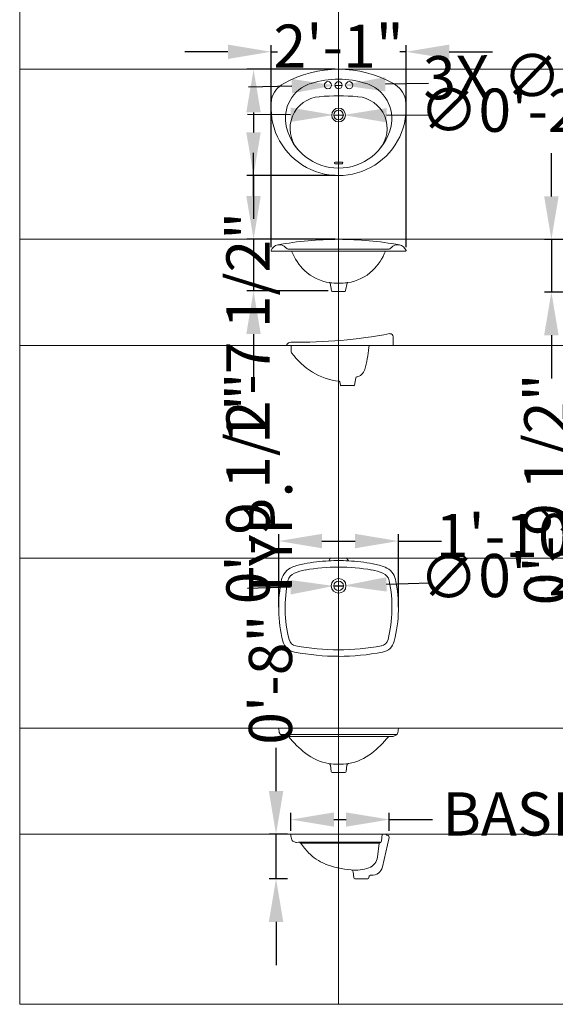
# Model space of a CAD drawing. Units: inches. Extents: x 2138 to 3265, y 2149 to 3392.
# Tile 7 of 13: x 2828 to 2928, y 3066 to 3248. Entities that reach past the tile are written whole.
import ezdxf

# ---------------------------------------------------------------- set-up
doc = ezdxf.new("R2010")
doc.units = ezdxf.units.IN
for name, color, linetype, lineweight in [('A-ANNO-DIMS', 2, 'Continuous', 18), ('A-DETL-GRID', 1, 'Continuous', 13), ('Washbasin-detail', 251, 'Continuous', 13), ('Washbasin-outline', 250, 'Continuous', 20)]:
    doc.layers.add(name, color=color, linetype=linetype, lineweight=lineweight)
doc.styles.get("Standard").update_dxf_attribs({"font": 'arial.ttf'})
doc.dimstyles.new('ISO-25', dxfattribs={"dimtxt": 8, "dimasz": 8, "dimexe": 1.25, "dimexo": 0.625, "dimtad": 0, "dimdec": 1, "dimlunit": 4, "dimtxsty": 'Standard', "dimcen": 2.5, "dimadec": 0, "dimazin": 0, "dimtfac": 1, "dimtdec": 1, "dimtmove": 0, "dimatfit": 3, "dimfxl": 1, "dimarcsym": 0})

# ---------------------------------------------------------------- blocks, each defined once
blk = doc.blocks.new('BASIN-WALLHUNG-SIDE')
for p, q in [((16.94, 8.23), (16.8, 6.96)), ((0.38, 6.97), (0.83, 6.75)), ((1.41, 6.77), (1.08, 6.71)), ((1.41, 6.77), (16.72, 6.77)), ((1.8, 6.61), (16.41, 6.61)), ((16.36, 6.61), (16.07, 4.02)), ((11.67, 0.17), (11.54, 1.3)), ((14.45, 0.17), (14.46, 0.29)), ((11.87, 0), (14.25, 0))]:
    blk.add_line(p, q)
for points in [[(17.61, 8.23), (0.08, 8.23, 0.427055), (0, 8.15, 0.060898), (0.18, 7.2)], [(17.81, 8.05), (18.01, 7.98, -0.38584), (18.2, 7.66), (16.99, 2.18)]]:
    blk.add_lwpolyline(points, format="xyb")
for centre, radius, start, end in [((17.61, 8.11), 0.119, 11.3189, 90), ((17.85, 8.16), 0.119, 191.3189, 251.9239), ((0.56, 7.33), 0.396, 197.6362, 243.4349), ((1.01, 7.1), 0.396, 243.4349, 279.8522), ((1.48, 6.38), 0.396, 36.3193, 99.8522), ((18.06, 18.57), 20.18, 216.3193, 223.028), ((16.41, 7.01), 0.396, 270, 353.6234), ((9.38, 10.47), 8.31, 223.028, 248.5761), ((13.71, 4.28), 2.37, 288.7646, 353.6234), ((12.27, 17.83), 16.23, 248.5761, 266.122), ((12.12, 7.8), 6.22, 261.2493, 292.2117), ((15.05, 2.61), 1.98, 265.1357, 347.5295), ((11.15, 1.25), 0.396, 6.7098, 86.122), ((11.87, 0.2), 0.198, 186.7098, 270), ((14.25, 0.2), 0.198, 270, 353.2902), ((14.85, 0.25), 0.396, 85.1357, 173.2902)]:
    blk.add_arc(centre, radius, start, end)
blk = doc.blocks.new('*D49')
at = {"layer": 'A-ANNO-DIMS', "color": 0, "lineweight": -2, "transparency": 16777216}
for p, q in [((2878.67, 3097.91), (2878.67, 3101.27)), ((2896.9, 3097.91), (2896.9, 3101.27)), ((2886.67, 3100.02), (2888.9, 3100.02)), ((2896.9, 3100.02), (2904.9, 3100.02))]:
    blk.add_line(p, q, dxfattribs=at)
at = {"layer": 'A-ANNO-DIMS', "color": 0, "transparency": 16777216}
for points in [[(2886.67, 3101.35), (2886.67, 3098.69), (2878.67, 3100.02)], [(2888.9, 3101.35), (2888.9, 3098.69), (2896.9, 3100.02)]]:
    blk.add_solid(points, dxfattribs=at)
at = {"layer": 'Defpoints', "color": 0, "transparency": 16777216}
for p in [(2896.9, 3100.02), (2878.67, 3097.29), (2896.9, 3097.29)]:
    blk.add_point(p, dxfattribs=at)
at = {"layer": 'A-ANNO-DIMS', "color": 0, "transparency": 16777216, "insert": (2948.05, 3100.02), "char_height": 8, "attachment_point": 5}
blk.add_mtext('BASIN 1\'-6" TYP.', dxfattribs=at)
blk = doc.blocks.new('*D50')
at = {"layer": 'A-ANNO-DIMS', "color": 0, "lineweight": -2, "transparency": 16777216}
for p, q in [((2875.94, 3105.29), (2875.94, 3113.29)), ((2878.04, 3097.29), (2874.69, 3097.29)), ((2875.94, 3089.06), (2875.94, 3097.29)), ((2878.04, 3089.06), (2874.69, 3089.06)), ((2875.94, 3081.06), (2875.94, 3073.06))]:
    blk.add_line(p, q, dxfattribs=at)
at = {"layer": 'A-ANNO-DIMS', "color": 0, "transparency": 16777216}
for points in [[(2874.6, 3105.29), (2877.27, 3105.29), (2875.94, 3097.29)], [(2874.6, 3081.06), (2877.27, 3081.06), (2875.94, 3089.06)]]:
    blk.add_solid(points, dxfattribs=at)
at = {"layer": 'Defpoints', "color": 0, "transparency": 16777216}
for p in [(2875.94, 3097.29), (2878.67, 3097.29), (2878.67, 3089.06)]:
    blk.add_point(p, dxfattribs=at)
at = {"layer": 'A-ANNO-DIMS', "color": 0, "transparency": 16777216, "insert": (2875.94, 3138.29), "char_height": 8, "attachment_point": 5, "rotation": 90}
blk.add_mtext('0\'-8" TYP.', dxfattribs=at)
blk = doc.blocks.new('*D79')
at = {"layer": 'A-ANNO-DIMS', "color": 0, "lineweight": -2, "transparency": 16777216}
for p, q in [((2875.02, 3206.04), (2875.02, 3243.52)), ((2900.02, 3206.04), (2900.02, 3243.52)), ((2867.02, 3242.27), (2859.02, 3242.27)), ((2875.02, 3242.27), (2876.19, 3242.27)), ((2900.02, 3242.27), (2898.84, 3242.27)), ((2908.02, 3242.27), (2916.02, 3242.27))]:
    blk.add_line(p, q, dxfattribs=at)
at = {"layer": 'A-ANNO-DIMS', "color": 0, "transparency": 16777216}
for points in [[(2867.02, 3243.6), (2867.02, 3240.94), (2875.02, 3242.27)], [(2908.02, 3243.6), (2908.02, 3240.94), (2900.02, 3242.27)]]:
    blk.add_solid(points, dxfattribs=at)
at = {"layer": 'Defpoints', "color": 0, "transparency": 16777216}
for p in [(2900.02, 3242.27), (2875.02, 3205.41), (2900.02, 3205.41)]:
    blk.add_point(p, dxfattribs=at)
at = {"layer": 'A-ANNO-DIMS', "color": 0, "transparency": 16777216, "insert": (2887.52, 3242.27), "char_height": 8, "attachment_point": 5}
blk.add_mtext('2\'-1"', dxfattribs=at)
blk = doc.blocks.new('*D80')
at = {"layer": 'A-ANNO-DIMS', "color": 0, "lineweight": -2, "transparency": 16777216}
for p, q in [((2886.89, 3239.02), (2870.52, 3239.02)), ((2871.77, 3231.02), (2871.77, 3227.33)), ((2886.89, 3219.33), (2870.52, 3219.33)), ((2871.77, 3219.33), (2871.77, 3211.33))]:
    blk.add_line(p, q, dxfattribs=at)
at = {"layer": 'A-ANNO-DIMS', "color": 0, "transparency": 16777216}
for points in [[(2870.43, 3231.02), (2873.1, 3231.02), (2871.77, 3239.02)], [(2870.43, 3227.33), (2873.1, 3227.33), (2871.77, 3219.33)]]:
    blk.add_solid(points, dxfattribs=at)
at = {"layer": 'Defpoints', "color": 0, "transparency": 16777216}
for p in [(2887.52, 3239.02), (2871.77, 3219.33), (2887.52, 3219.33)]:
    blk.add_point(p, dxfattribs=at)
at = {"layer": 'A-ANNO-DIMS', "color": 0, "transparency": 16777216, "insert": (2871.77, 3191.13), "char_height": 8, "attachment_point": 5, "rotation": 90}
blk.add_mtext('1\'-7 1/2"', dxfattribs=at)
blk = doc.blocks.new('*D81')
at = {"layer": 'A-ANNO-DIMS', "color": 0, "lineweight": -2, "transparency": 16777216}
for p, q in [((2871.77, 3215.52), (2871.77, 3223.52)), ((2886.89, 3207.52), (2870.52, 3207.52)), ((2871.77, 3207.52), (2871.77, 3197.95)), ((2885.61, 3197.95), (2870.52, 3197.95)), ((2871.77, 3189.95), (2871.77, 3181.95))]:
    blk.add_line(p, q, dxfattribs=at)
at = {"layer": 'A-ANNO-DIMS', "color": 0, "transparency": 16777216}
for points in [[(2870.43, 3215.52), (2873.1, 3215.52), (2871.77, 3207.52)], [(2870.43, 3189.95), (2873.1, 3189.95), (2871.77, 3197.95)]]:
    blk.add_solid(points, dxfattribs=at)
at = {"layer": 'Defpoints', "color": 0, "transparency": 16777216}
for p in [(2887.52, 3207.52), (2871.77, 3197.95), (2886.23, 3197.95)]:
    blk.add_point(p, dxfattribs=at)
at = {"layer": 'A-ANNO-DIMS', "color": 0, "transparency": 16777216, "insert": (2871.77, 3161.38), "char_height": 8, "attachment_point": 5, "rotation": 90}
blk.add_mtext('0\'-9 1/2"', dxfattribs=at)
blk = doc.blocks.new('*D83')
at = {"layer": 'A-ANNO-DIMS', "color": 0, "lineweight": -2, "transparency": 16777216}
for p, q in [((2926.93, 3215.47), (2926.93, 3223.47)), ((2930.28, 3207.47), (2925.68, 3207.47)), ((2926.93, 3207.47), (2926.93, 3197.76)), ((2946.5, 3197.76), (2925.68, 3197.76)), ((2926.93, 3189.76), (2926.93, 3181.76))]:
    blk.add_line(p, q, dxfattribs=at)
at = {"layer": 'A-ANNO-DIMS', "color": 0, "transparency": 16777216}
for points in [[(2925.59, 3215.47), (2928.26, 3215.47), (2926.93, 3207.47)], [(2925.59, 3189.76), (2928.26, 3189.76), (2926.93, 3197.76)]]:
    blk.add_solid(points, dxfattribs=at)
at = {"layer": 'Defpoints', "color": 0, "transparency": 16777216}
for p in [(2930.91, 3207.47), (2926.93, 3197.76), (2947.13, 3197.76)]:
    blk.add_point(p, dxfattribs=at)
at = {"layer": 'A-ANNO-DIMS', "color": 0, "transparency": 16777216, "insert": (2926.93, 3161.18), "char_height": 8, "attachment_point": 5, "rotation": 90}
blk.add_mtext('0\'-9 1/2"', dxfattribs=at)
blk = doc.blocks.new('*D97')
at = {"layer": 'A-ANNO-DIMS', "color": 0, "lineweight": -2, "transparency": 16777216}
for p, q in [((2876.44, 3139.39), (2876.44, 3152.87)), ((2898.59, 3139.39), (2898.59, 3152.87)), ((2884.44, 3151.62), (2890.59, 3151.62)), ((2898.59, 3151.62), (2906.59, 3151.62))]:
    blk.add_line(p, q, dxfattribs=at)
at = {"layer": 'A-ANNO-DIMS', "color": 0, "transparency": 16777216}
for points in [[(2884.44, 3152.95), (2884.44, 3150.28), (2876.44, 3151.62)], [(2890.59, 3152.95), (2890.59, 3150.28), (2898.59, 3151.62)]]:
    blk.add_solid(points, dxfattribs=at)
at = {"layer": 'Defpoints', "color": 0, "transparency": 16777216}
for p in [(2898.59, 3151.62), (2876.44, 3138.77), (2898.59, 3138.77)]:
    blk.add_point(p, dxfattribs=at)
at = {"layer": 'A-ANNO-DIMS', "color": 0, "transparency": 16777216, "insert": (2920.58, 3151.62), "char_height": 8, "attachment_point": 5}
blk.add_mtext('1\'-10"', dxfattribs=at)
blk = doc.blocks.new('*D121')
at = {"layer": 'A-ANNO-DIMS', "color": 0, "lineweight": -2, "transparency": 16777216}
for p, q in [((2904.18, 3236.4), (2896.19, 3236.24)), ((2878.85, 3235.89), (2870.85, 3235.74)), ((2886.85, 3236.05), (2888.19, 3236.08))]:
    blk.add_line(p, q, dxfattribs=at)
at = {"layer": 'A-ANNO-DIMS', "color": 0, "transparency": 16777216}
for points in [[(2878.82, 3237.23), (2878.88, 3234.56), (2886.85, 3236.05)], [(2896.16, 3237.57), (2896.21, 3234.91), (2888.19, 3236.08)]]:
    blk.add_solid(points, dxfattribs=at)
at = {"layer": 'Defpoints', "color": 0, "transparency": 16777216}
for p in [(2886.85, 3236.05), (2888.19, 3236.08)]:
    blk.add_point(p, dxfattribs=at)
at = {"layer": 'A-ANNO-DIMS', "color": 0, "transparency": 16777216, "insert": (2937.49, 3237.06), "char_height": 8, "attachment_point": 5, "rotation": 1.1379}
blk.add_mtext('3X ∅0\'-1 1/2"', dxfattribs=at)
blk = doc.blocks.new('*D122')
at = {"layer": 'A-ANNO-DIMS', "color": 0, "lineweight": -2, "transparency": 16777216}
for p, q in [((2878.63, 3230.6), (2870.63, 3230.64)), ((2886.63, 3230.56), (2888.4, 3230.55)), ((2904.4, 3230.47), (2896.4, 3230.51))]:
    blk.add_line(p, q, dxfattribs=at)
at = {"layer": 'A-ANNO-DIMS', "color": 0, "transparency": 16777216}
for points in [[(2878.64, 3231.93), (2878.63, 3229.27), (2886.63, 3230.56)], [(2896.41, 3231.84), (2896.4, 3229.18), (2888.4, 3230.55)]]:
    blk.add_solid(points, dxfattribs=at)
at = {"layer": 'Defpoints', "color": 0, "transparency": 16777216}
for p in [(2886.63, 3230.56), (2888.4, 3230.55)]:
    blk.add_point(p, dxfattribs=at)
at = {"layer": 'A-ANNO-DIMS', "color": 0, "transparency": 16777216, "insert": (2920.01, 3230.39), "char_height": 8, "attachment_point": 5, "rotation": 359.7153}
blk.add_mtext('∅0\'-2"', dxfattribs=at)
blk = doc.blocks.new('*D130')
at = {"layer": 'A-ANNO-DIMS', "color": 0, "lineweight": -2, "transparency": 16777216}
for p, q in [((2886.63, 3143.3), (2888.41, 3143.35)), ((2904.4, 3143.83), (2896.4, 3143.59)), ((2878.63, 3143.06), (2870.63, 3142.82))]:
    blk.add_line(p, q, dxfattribs=at)
at = {"layer": 'A-ANNO-DIMS', "color": 0, "transparency": 16777216}
for points in [[(2878.59, 3144.39), (2878.67, 3141.72), (2886.63, 3143.3)], [(2896.36, 3144.92), (2896.44, 3142.26), (2888.41, 3143.35)]]:
    blk.add_solid(points, dxfattribs=at)
at = {"layer": 'Defpoints', "color": 0, "transparency": 16777216}
for p in [(2886.63, 3143.3), (2888.41, 3143.35)]:
    blk.add_point(p, dxfattribs=at)
at = {"layer": 'A-ANNO-DIMS', "color": 0, "transparency": 16777216, "insert": (2920, 3144.3), "char_height": 8, "attachment_point": 5, "rotation": 1.7228}
blk.add_mtext('∅0\'-2"', dxfattribs=at)

msp = doc.modelspace()

# ---------------------------------------------------------------- linework, layer by layer
at = {"layer": 'A-DETL-GRID'}
for p, q in [((2828.46, 3239.02), (2828.46, 3370.91)), ((2887.52, 3239.02), (2887.52, 3370.91)), ((2828.46, 3239.02), (3241.85, 3239.02)), ((2828.46, 3239.02), (3241.85, 3239.02)), ((2828.46, 3148.47), (2828.46, 3239.02)), ((2887.52, 3148.47), (2887.52, 3239.02)), ((2828.46, 3207.52), (3241.85, 3207.52)), ((2828.46, 3187.84), (3241.85, 3187.84)), ((2828.46, 3148.47), (3241.85, 3148.47)), ((2828.46, 3148.47), (3241.85, 3148.47)), ((2828.46, 3065.79), (2828.46, 3148.47)), ((2887.52, 3065.79), (2887.52, 3148.47)), ((2828.46, 3116.97), (3241.85, 3116.97)), ((2828.46, 3097.29), (3241.85, 3097.29)), ((2828.46, 3065.79), (3241.85, 3065.79))]:
    msp.add_line(p, q, dxfattribs=at)
at = {"layer": 'Washbasin-detail'}
for p, q in [((2886.88, 3221.82), (2887.52, 3221.82)), ((2888.16, 3221.82), (2887.52, 3221.82)), ((2886.88, 3221.52), (2887.52, 3221.52)), ((2888.16, 3221.52), (2887.52, 3221.52)), ((2878.72, 3187.84), (2893.48, 3187.84)), ((2887.52, 3115.78), (2876.72, 3115.78)), ((2887.52, 3115.78), (2898.32, 3115.78))]:
    msp.add_line(p, q, dxfattribs=at)
for centre, radius in [((2885.55, 3236.07), 0.669), ((2887.52, 3236.07), 0.669), ((2889.49, 3236.07), 0.669), ((2887.52, 3230.55), 1.28), ((2887.52, 3230.55), 0.886), ((2887.52, 3143.32), 1.37), ((2887.52, 3143.32), 0.89)]:
    msp.add_circle(centre, radius, dxfattribs=at)
for centre, radius, start, end in [((2884.45, 3228.05), 5.92, 94.5762, 220.138), ((2887.52, 3189.71), 44.39, 85.4238, 94.5762), ((2890.59, 3228.05), 5.92, 319.862, 85.4238), ((2886.88, 3221.67), 0.146, 90, 270), ((2888.16, 3221.67), 0.146, 270, 90), ((2887.52, 3145.54), 61.98, 90, 100.4767), ((2887.52, 3145.54), 61.98, 79.5233, 90), ((2887.52, 3213.85), 14.46, 263.4006, 276.5994), ((2887.52, 3112.38), 34.43, 90, 100.3055), ((2887.52, 3112.38), 34.43, 79.6945, 90), ((2880.08, 3143.84), 1.98, 111.509, 168.1174), ((2883.27, 3135.74), 10.69, 100.3055, 111.509), ((2891.77, 3135.74), 10.69, 68.491, 79.6945), ((2894.96, 3143.84), 1.98, 11.8826, 68.491), ((2901.76, 3139.27), 24.14, 168.1174, 194.1676), ((2873.27, 3139.27), 24.14, 345.8324, 11.8826), ((2879.89, 3133.75), 1.58, 194.1676, 259.2192), ((2887.52, 3173.8), 42.34, 259.2192, 270), ((2887.52, 3173.8), 42.34, 270, 280.7808), ((2895.14, 3133.75), 1.58, 280.7808, 345.8324), ((2887.25, 3119.78), 9.5, 260.4365, 271.6387), ((2887.79, 3119.78), 9.5, 268.3613, 279.5635)]:
    msp.add_arc(centre, radius, start, end, dxfattribs=at)
at = {"layer": 'Washbasin-outline'}
for p, q in [((2878.83, 3205.31), (2875.14, 3205.31)), ((2887.52, 3205.7), (2878.35, 3205.7)), ((2887.52, 3205.31), (2878.83, 3205.31)), ((2887.52, 3205.7), (2896.69, 3205.7)), ((2887.52, 3205.31), (2896.2, 3205.31)), ((2896.2, 3205.31), (2899.9, 3205.31)), ((2885.96, 3199.4), (2886.21, 3198.01)), ((2887.52, 3197.88), (2886.37, 3197.88)), ((2886.37, 3197.88), (2887.52, 3197.88)), ((2888.67, 3197.88), (2887.52, 3197.88)), ((2887.52, 3197.88), (2888.67, 3197.88)), ((2889.08, 3199.4), (2888.82, 3198.01)), ((2897.62, 3189.44), (2897.62, 3187.84)), ((2897.62, 3187.84), (2897.62, 3189.44)), ((2878.05, 3187.84), (2878.72, 3187.84)), ((2878.79, 3188.47), (2878.68, 3188.47)), ((2878.72, 3187.84), (2878.72, 3186.86)), ((2893.48, 3187.84), (2897.62, 3187.84)), ((2890.71, 3181.89), (2890.45, 3180.47)), ((2887.75, 3181.1), (2887.86, 3180.47)), ((2887.94, 3180.41), (2890.37, 3180.41)), ((2887.94, 3180.41), (2890.37, 3180.41)), ((2885.71, 3147.95), (2885.99, 3148.38)), ((2888.88, 3148.47), (2886.16, 3148.47)), ((2889.33, 3147.95), (2889.04, 3148.38)), ((2876.52, 3116.97), (2887.52, 3116.97)), ((2898.52, 3116.97), (2887.52, 3116.97)), ((2876.82, 3115.71), (2877.3, 3115.47)), ((2878.23, 3115.43), (2877.48, 3115.43)), ((2887.52, 3115.43), (2878.23, 3115.43)), ((2887.52, 3115.43), (2896.75, 3115.43)), ((2896.8, 3115.43), (2897.56, 3115.43)), ((2898.22, 3115.71), (2897.73, 3115.47)), ((2886.13, 3108.92), (2886, 3110.07)), ((2886.33, 3108.74), (2887.52, 3108.74)), ((2888.71, 3108.74), (2887.52, 3108.74)), ((2888.9, 3108.92), (2889.04, 3110.07))]:
    msp.add_line(p, q, dxfattribs=at)
msp.add_lwpolyline([(2887.52, 3130.26, 0.047075), (2895.66, 3131.03, 0.291718), (2897.83, 3133.08, 0.114157), (2898.06, 3144.49)], format="xyb", dxfattribs=at)
for centre, radius, start, end in [((2887.52, 3217.95), 21.07, 61.2064, 118.7936), ((2879.56, 3232.42), 4.56, 118.7936, 167.1119), ((2884.5, 3229.9), 6.84, 107.4348, 193.7987), ((2887.52, 3220.3), 16.89, 72.5652, 107.4348), ((2890.53, 3229.9), 6.84, 346.2013, 72.5652), ((2895.47, 3232.42), 4.56, 12.8881, 61.2064), ((2887.52, 3231.83), 12.5, 172.6336, 7.3664), ((2887.52, 3230.64), 9.94, 193.7987, 346.2013), ((2876.54, 3204.89), 1.62, 100.4767, 159.2184), ((2875.14, 3205.43), 0.118, 159.2184, 270), ((2876.54, 3204.89), 1.62, 41.4973, 100.4767), ((2878.35, 3206.49), 0.787, 221.4973, 270), ((2888.34, 3209.1), 10.24, 201.7293, 226.0695), ((2886.69, 3209.1), 10.24, 313.9305, 338.2707), ((2896.69, 3206.49), 0.787, 270, 318.5027), ((2898.49, 3204.89), 1.62, 79.5233, 138.5027), ((2898.49, 3204.89), 1.62, 20.7816, 79.5233), ((2899.9, 3205.43), 0.118, 270, 20.7816), ((2886.97, 3207.69), 8.27, 226.1071, 262.2475), ((2888.06, 3207.69), 8.27, 277.7525, 313.8929), ((2885.84, 3199.38), 0.118, 10.4455, 82.2475), ((2886.37, 3198.03), 0.157, 190.4455, 270), ((2888.67, 3198.03), 0.157, 270, 349.5545), ((2889.19, 3199.38), 0.118, 97.7525, 169.5545), ((2880.11, 3279.13), 90.67, 269.163, 280.7441), ((2897.02, 3189.44), 0.602, 0, 90), ((2878.05, 3187.96), 0.118, 150.4596, 270), ((2878.72, 3187.58), 0.887, 89.9487, 150.4596), ((2874.63, 3188.67), 18.5, 343.3947, 356.2685), ((2893.48, 3187.44), 0.394, 90, 176.2685), ((2879.31, 3186.86), 0.591, 180, 214.8973), ((2889.16, 3193.73), 12.6, 214.8973, 263.017), ((2890.47, 3183.95), 1.97, 280.2886, 343.3947), ((2890.86, 3181.86), 0.157, 99.8181, 169.5011), ((2887.59, 3181.07), 0.157, 10.4989, 76.25), ((2887.94, 3180.48), 0.0787, 190.4989, 270), ((2890.37, 3180.48), 0.0787, 270, 349.5011), ((2880.08, 3143.84), 3.17, 111.509, 168.1174), ((2883.27, 3135.74), 11.87, 100.3055, 111.509), ((2887.52, 3112.38), 35.62, 92.9155, 100.3055), ((2887.52, 3112.38), 35.62, 90, 92.9155), ((2886.16, 3148.27), 0.198, 90, 146.3099), ((2887.52, 3112.38), 35.62, 87.0845, 90), ((2888.88, 3148.27), 0.198, 33.6901, 90), ((2887.52, 3112.38), 35.62, 79.6945, 87.0845), ((2891.77, 3135.74), 11.87, 68.491, 79.6945), ((2894.96, 3143.84), 3.17, 11.8826, 68.491), ((2901.76, 3139.27), 25.33, 168.1174, 194.1676), ((2879.89, 3133.75), 2.77, 194.1676, 259.2192), ((2887.52, 3173.8), 43.53, 259.2192, 270), ((2876.52, 3116.89), 0.0791, 90, 183.9922), ((2876.52, 3116.89), 0.0791, 90, 183.9922), ((2880.38, 3117.16), 3.96, 183.9922, 197.9317), ((2877, 3116.07), 0.396, 197.9317, 243.4349), ((2898.04, 3116.07), 0.396, 296.5651, 342.0683), ((2894.65, 3117.16), 3.96, 342.0683, 356.0078), ((2898.52, 3116.89), 0.0791, 356.0078, 90), ((2898.52, 3116.89), 0.0791, 356.0078, 90), ((2877.48, 3115.82), 0.396, 243.4349, 270), ((2893.23, 3127.44), 19.22, 218.6937, 232.1175), ((2882.22, 3126.98), 18.6, 307.7469, 321.3924), ((2897.06, 3115.13), 0.396, 130.7889, 141.3924), ((2897.56, 3115.82), 0.396, 270, 296.5651), ((2887.25, 3119.78), 9.5, 232.2531, 260.4365), ((2887.79, 3119.78), 9.5, 279.5635, 307.7469), ((2885.6, 3110.03), 0.396, 6.7098, 80.4365), ((2889.43, 3110.03), 0.396, 99.5635, 173.2902), ((2886.33, 3108.94), 0.198, 186.7098, 270), ((2888.71, 3108.94), 0.198, 270, 353.2902)]:
    msp.add_arc(centre, radius, start, end, dxfattribs=at)

# ---------------------------------------------------------------- block references
msp.add_blockref('BASIN-WALLHUNG-SIDE', (2878.67, 3089.06), dxfattribs=at)

# ---------------------------------------------------------------- dimensions: what is measured, and where the dimension line sits
at = {"layer": 'A-ANNO-DIMS'}
dim = msp.add_diameter_dim_2p(p1=(2886.85, 3236.05), p2=(2888.19, 3236.08), text='3X <>', dimstyle='ISO-25', override={"dimdec": 1, "dimlfac": 1, "dimrnd": 0, "dimzin": 1, "dimdsep": 46, "dimlunit": 4, "dimfrac": 2}, dxfattribs=at)
dim.commit()
dim.dimension.update_dxf_attribs({"geometry": '*D121', "text_midpoint": (2937.49, 3237.06), "dimtype": 163})
for base, p1, p2, picture, middle in [((2900.02, 3242.27), (2875.02, 3205.41), (2900.02, 3205.41), '*D79', (2887.52, 3242.27)), ((2898.5936, 3151.6182), (2876.4419, 3138.7697), (2898.5936, 3138.7697), '*D97', (2920.5829, 3151.6182))]:
    dim = msp.add_linear_dim(base=base, p1=p1, p2=p2, dimstyle='ISO-25', override={"dimdec": 1, "dimlfac": 1, "dimrnd": 0, "dimzin": 1, "dimdsep": 46, "dimlunit": 4, "dimfrac": 2}, dxfattribs=at)
    dim.commit()
    dim.dimension.update_dxf_attribs({"geometry": picture, "text_midpoint": middle})
for base, p1, p2, picture, middle in [((2871.77, 3219.33), (2887.52, 3239.02), (2887.52, 3219.33), '*D80', (2871.77, 3191.13)), ((2871.77, 3197.95), (2887.52, 3207.52), (2886.23, 3197.95), '*D81', (2871.77, 3161.38)), ((2926.93, 3197.76), (2930.91, 3207.47), (2947.13, 3197.76), '*D83', (2926.93, 3161.18))]:
    dim = msp.add_linear_dim(base=base, p1=p1, p2=p2, angle=90, dimstyle='ISO-25', override={"dimdec": 1, "dimlfac": 1, "dimrnd": 0, "dimzin": 1, "dimdsep": 46, "dimlunit": 4, "dimfrac": 2}, dxfattribs=at)
    dim.commit()
    dim.dimension.update_dxf_attribs({"geometry": picture, "text_midpoint": middle})
for p1, p2, picture, middle in [((2886.63, 3230.56), (2888.4, 3230.55), '*D122', (2920.01, 3230.39)), ((2886.63, 3143.3), (2888.41, 3143.35), '*D130', (2920, 3144.3))]:
    dim = msp.add_diameter_dim_2p(p1=p1, p2=p2, dimstyle='ISO-25', override={"dimdec": 1, "dimlfac": 1, "dimrnd": 0, "dimzin": 1, "dimdsep": 46, "dimlunit": 4, "dimfrac": 2}, dxfattribs=at)
    dim.commit()
    dim.dimension.update_dxf_attribs({"geometry": picture, "text_midpoint": middle})
dim = msp.add_linear_dim(base=(2875.94, 3097.29), p1=(2878.67, 3089.06), p2=(2878.67, 3097.29), angle=90, text='<> TYP.', dimstyle='ISO-25', override={"dimdec": 1, "dimlfac": 1, "dimrnd": 0, "dimzin": 1, "dimdsep": 46, "dimlunit": 4, "dimfrac": 2}, dxfattribs=at)
dim.commit()
dim.dimension.update_dxf_attribs({"geometry": '*D50', "text_midpoint": (2875.94, 3138.29)})
dim = msp.add_linear_dim(base=(2896.9, 3100.02), p1=(2878.67, 3097.29), p2=(2896.9, 3097.29), text='BASIN <> TYP.', dimstyle='ISO-25', override={"dimdec": 1, "dimlfac": 1, "dimrnd": 0, "dimzin": 1, "dimdsep": 46, "dimlunit": 4, "dimfrac": 2}, dxfattribs=at)
dim.commit()
dim.dimension.update_dxf_attribs({"geometry": '*D49', "text_midpoint": (2948.05, 3100.02)})

doc.saveas('drawing.dxf')
